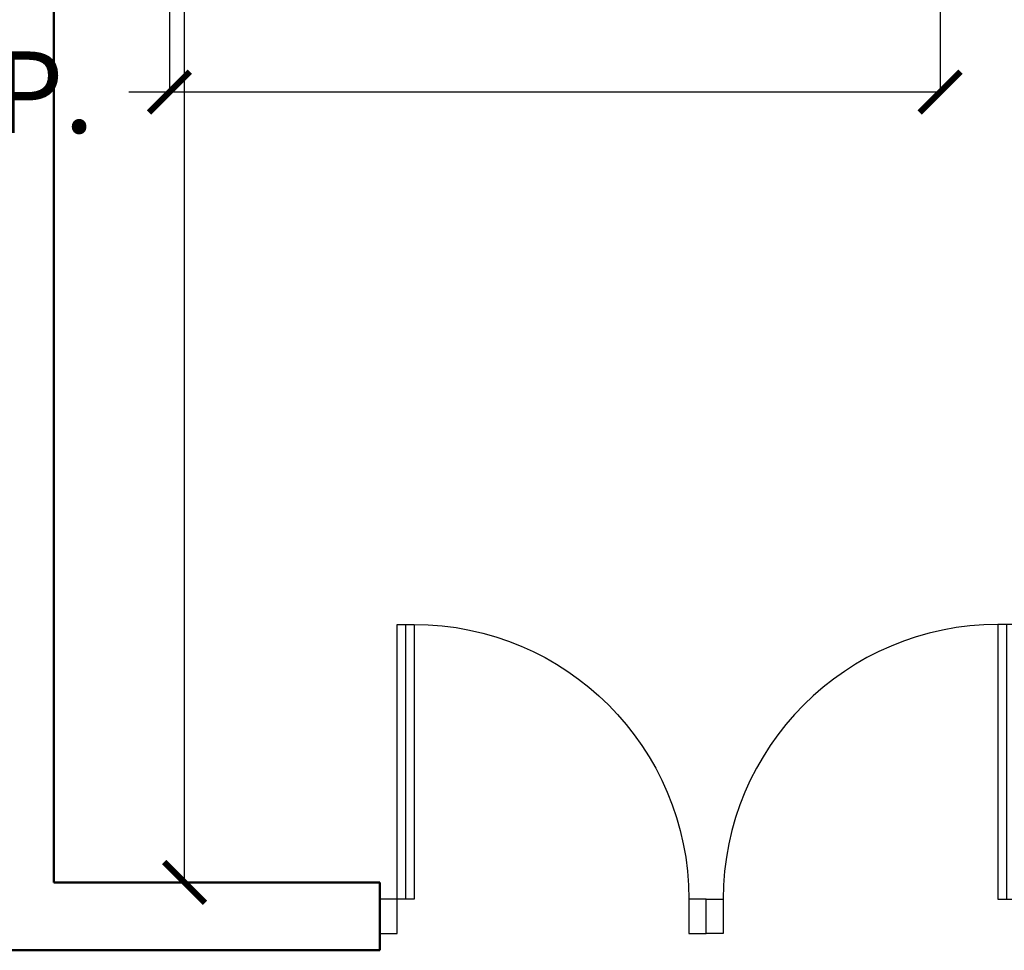
# Model space of a CAD drawing. Units: inches. Extents: x 147 to 1638, y 107 to 941.
# Tile 5 of 17: x 469 to 542, y 247 to 315. Entities that reach past the tile are written whole.
import ezdxf

# ---------------------------------------------------------------- set-up
doc = ezdxf.new("R2010")
doc.units = ezdxf.units.IN
doc.header["$MEASUREMENT"] = 0
for name, color, linetype, lineweight in [('A-ANNO-DIMS', 2, 'Continuous', 15), ('A-Door', 150, 'Continuous', 25), ('walls', 7, 'Continuous', 50)]:
    doc.layers.add(name, color=color, linetype=linetype, lineweight=lineweight)
doc.layers.add('A-Glaz', color=92, linetype='Continuous')
doc.layers.add('NT', color=1, linetype='Continuous')
doc.styles.get("Standard").update_dxf_attribs({"font": 'arial.ttf'})
doc.dimstyles.get("Standard").update_dxf_attribs({"dimtxt": 6, "dimasz": 3, "dimexe": 0.18, "dimexo": 0.0625, "dimgap": 0.09, "dimtad": 0, "dimtih": 1, "dimtoh": 1, "dimdec": 1, "dimzin": 0, "dimdsep": 46, "dimlunit": 3, "dimtxsty": 'Standard', "dimblk": 'ARCHTICK', "dimcen": 0.09, "dimadec": 0, "dimazin": 0, "dimtfac": 1, "dimtdec": 1, "dimtofl": 0, "dimtmove": 0, "dimatfit": 3, "dimfxl": 1, "dimtolj": 1, "dimtzin": 0, "dimarcsym": 0})

# ---------------------------------------------------------------- blocks, each defined once
blk = doc.blocks.new('A$C087A3AA9')
at = {"layer": 'A-Door'}
for points in [[(852.6, 94.7), (852.6, 852.6), (805.3, 852.6), (805.3, 94.7)], [(47.4, 94.7), (47.4, 0), (0, 0), (0, 94.7)], [(900, 94.7), (900, 0), (852.6, 0), (852.6, 94.7)]]:
    blk.add_lwpolyline(points, close=True, dxfattribs=at)
at = {"layer": 'A-Glaz'}
blk.add_line((828.9, 852.6), (828.9, 94.7), dxfattribs=at)
at = {"layer": 'NT'}
blk.add_arc((805.3, 94.7), 757.9, 90, 180, dxfattribs=at)
blk = doc.blocks.new('_ArchTick')
at = {"color": 0, "linetype": 'ByBlock', "const_width": 0.15}
blk.add_lwpolyline([(-0.5, -0.5), (0.5, 0.5)], dxfattribs=at)
blk = doc.blocks.new('*D28')
at = {"layer": 'A-ANNO-DIMS', "color": 0, "lineweight": -2, "transparency": 16777216}
for p, q in [((483.882, 395.718), (481.394, 395.718)), ((481.574, 395.718), (481.574, 326.82)), ((481.574, 251.718), (481.574, 320.616)), ((483.882, 251.718), (481.394, 251.718))]:
    blk.add_line(p, q, dxfattribs=at)
at = {"layer": 'Defpoints', "color": 0, "lineweight": -2, "transparency": 16777216}
for p in [(483.944, 395.718), (481.574, 251.718), (483.944, 251.718)]:
    blk.add_point(p, dxfattribs=at)
at = {"layer": 'A-ANNO-DIMS', "color": 0, "lineweight": -2, "transparency": 16777216, "xscale": 3, "yscale": 3, "zscale": 3}
for p, rotation in [((481.574, 395.718), 90), ((481.574, 251.718), 270)]:
    blk.add_blockref('_ArchTick', p, dxfattribs=dict(at, rotation=rotation))
at = {"layer": 'A-ANNO-DIMS', "color": 0, "transparency": 16777216, "insert": (481.574, 323.718), "char_height": 6, "attachment_point": 5}
blk.add_mtext("\\A1;12'", dxfattribs=at)
blk = doc.blocks.new('*D116')
at = {"layer": 'A-ANNO-DIMS', "color": 0, "lineweight": -2, "transparency": 16777216}
for p, q in [((480.463, 318.293), (480.463, 309.67)), ((537.162, 318.293), (537.162, 309.67)), ((480.463, 309.85), (477.463, 309.85)), ((537.162, 309.85), (480.463, 309.85))]:
    blk.add_line(p, q, dxfattribs=at)
at = {"layer": 'Defpoints', "color": 0, "lineweight": -2, "transparency": 16777216}
for p in [(480.463, 318.355), (537.162, 318.355), (480.463, 309.85)]:
    blk.add_point(p, dxfattribs=at)
at = {"layer": 'A-ANNO-DIMS', "color": 0, "lineweight": -2, "transparency": 16777216, "xscale": 3, "yscale": 3, "zscale": 3, "rotation": 180}
blk.add_blockref('_ArchTick', (480.463, 309.85), dxfattribs=at)
at = {"layer": 'A-ANNO-DIMS', "color": 0, "lineweight": -2, "transparency": 16777216, "xscale": 3, "yscale": 3, "zscale": 3}
blk.add_blockref('_ArchTick', (537.162, 309.85), dxfattribs=at)
at = {"layer": 'A-ANNO-DIMS', "color": 0, "transparency": 16777216, "insert": (430.22, 309.85), "char_height": 6, "attachment_point": 5}
blk.add_mtext('\\A1;SOFA SET 4\'-8 1/2" TYP.', dxfattribs=at)

msp = doc.modelspace()

# ---------------------------------------------------------------- linework, layer by layer
at = {"layer": 'walls'}
for p, q in [((471.944, 395.718), (471.944, 251.718)), ((471.944, 251.718), (495.944, 251.718)), ((495.944, 251.718), (495.944, 246.718)), ((466.944, 246.718), (495.944, 246.718))]:
    msp.add_line(p, q, dxfattribs=at)

# ---------------------------------------------------------------- block references
at = {"layer": 'A-Door', "yscale": 0.0266666667542921, "zscale": 0.0266666667542921}
for xscale in [-0.0266666667542921, 0.0266666667542921]:
    msp.add_blockref('A$C087A3AA9', (519.944, 247.955), dxfattribs=dict(at, xscale=xscale))

# ---------------------------------------------------------------- dimensions: what is measured, and where the dimension line sits
at = {"layer": 'A-ANNO-DIMS'}
dim = msp.add_linear_dim(base=(481.574, 251.718), p1=(483.944, 395.718), p2=(483.944, 251.718), angle=90, dimstyle='Standard', override={"dimclrd": 0, "dimclre": 0, "dimclrt": 0}, dxfattribs=at)
dim.commit()
dim.dimension.update_dxf_attribs({"geometry": '*D28', "text_midpoint": (481.574, 323.718)})
dim = msp.add_linear_dim(base=(480.463, 309.85), p1=(537.162, 318.355), p2=(480.463, 318.355), angle=180, text='SOFA SET <> TYP.', dimstyle='Standard', override={"dimdec": 1, "dimlfac": 1, "dimrnd": 0, "dimzin": 1, "dimdsep": 46, "dimlunit": 4, "dimfrac": 2}, dxfattribs=at)
dim.commit()
dim.dimension.update_dxf_attribs({"geometry": '*D116', "text_midpoint": (430.22, 309.85)})

doc.saveas('drawing.dxf')
